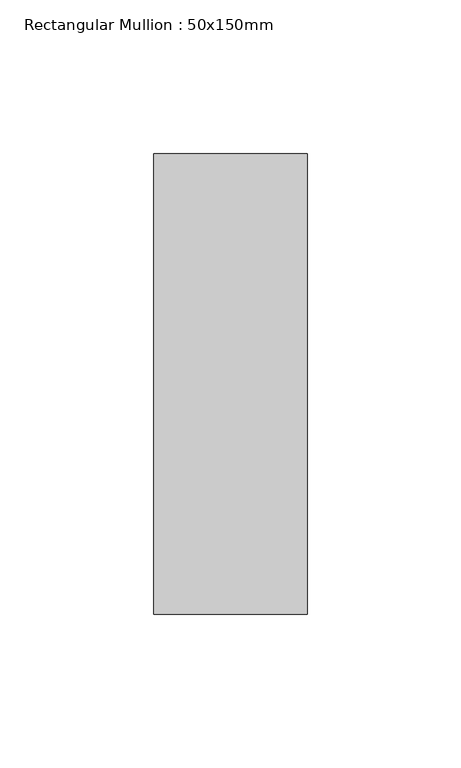
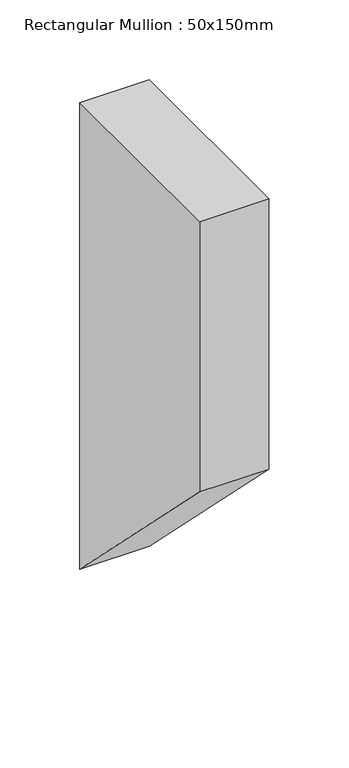
"""IFC4 building model written with IfcOpenShell, lengths in millimetres: member geometry, Rectangular Mullion : 50x150mm."""

from ifc_helpers import new_model, si_unit, frame, origin, place, context, project, spatial, polyline, outline, extrude, source, transform, mapped, element, save


def rectangular_mullion_50x150mm_3c996cd3(model_context):
    return source(origin(), model_context, "Body", "SweptSolid", [
        extrude(outline(polyline([(-75.0, 0.0), (75.0, 0.0), (75.0, -356.5166667), (-75.0, -206.5166667), (-75.0, 0.0)])), frame((-50.0, 0.0, 0.0), z_axis=(1.0, 0.0, 0.0), x_axis=(0.0, 1.0, 0.0)), (0.0, 0.0, 1.0), 50.0),
    ])


if __name__ == "__main__":
    model = new_model("IFC4")
    model_context = context("Model", 3, world=origin())
    ifc_project = project(units=[si_unit("LENGTHUNIT", "METRE", prefix="MILLI")], contexts=[model_context])
    site = spatial("IfcSite", under=ifc_project)
    building = spatial("IfcBuilding", under=site)
    placement = place(None, origin())
    rectangular_mullion_50x150mm_shape = rectangular_mullion_50x150mm_3c996cd3(model_context)
    element("IfcMember", 1, ObjectType="Rectangular Mullion : 50x150mm", at=placement, inside=building, context=model_context, shape_type="MappedRepresentation", body=[
        mapped(rectangular_mullion_50x150mm_shape, transform((0.0, 0.0, 0.0), x_axis=(1.0, 0.0, 0.0), y_axis=(0.0, 1.0, 0.0), z_axis=(0.0, 0.0, 1.0))),
    ])
    save(model, "model.ifc")

# Revit data of these elements
# Type "Rectangular Mullion : 50x150mm"
#   Keynote = "H11"
#   built-in parameter 1007304 = 0.492126 (stored number, unit not read)
#   built-in parameter 1007301 = 0.082021 (stored number, unit not read)
#   built-in parameter 1007300 = 0.082021 (stored number, unit not read)
# Element 1 (IfcMember, "Rectangular Mullion : 50x150mm")
#   Materials on its faces: "Aluminium"
# Materials
#   "Aluminium": class "Metal", colour RGB 247 247 247, transparency 0, Description = "Aluminium 6061", Cost = 0
